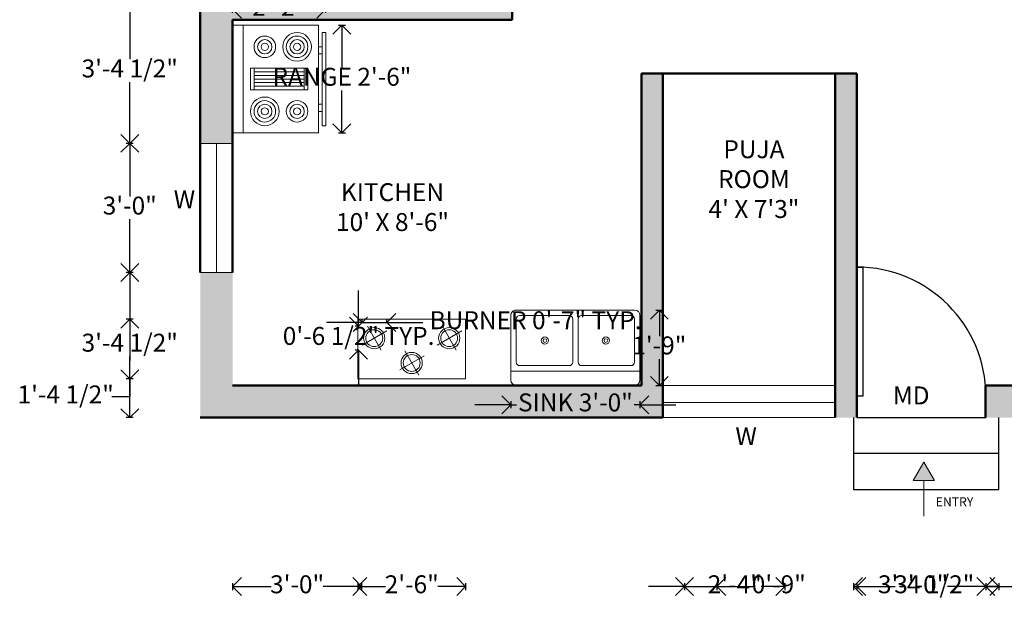
# Model space of a CAD drawing. Units: inches. Extents: x 2691 to 3149, y 584 to 962.
# Tile 1 of 3: x 2691 to 2966, y 584 to 750. Entities that reach past the tile are written whole.
import ezdxf

# ---------------------------------------------------------------- set-up
doc = ezdxf.new("R2010")
doc.units = ezdxf.units.IN
for name, color, linetype, lineweight in [('A-ANNO-DIMS', 2, 'Continuous', 18), ('A-ANNO-SYMB', 252, 'Continuous', 18), ('A-ANNO-TEXT', 159, 'Continuous', 18), ('A-AREA-IDEN', 7, 'Continuous', 25), ('A-DOOR', 4, 'Continuous', 25), ('A-EQPM', 8, 'Continuous', 18), ('A-FLOR-FIXT', 9, 'Continuous', 18), ('A-FLOR-STRS', 7, 'Continuous', 25), ('A-GLAZ', 40, 'Continuous', 18), ('A-WALL', 254, 'Continuous', 50), ('A-WALL-PATT', 252, 'Continuous', 13)]:
    doc.layers.add(name, color=color, linetype=linetype, lineweight=lineweight)
doc.styles.get("Standard").update_dxf_attribs({"font": 'arial.ttf'})
doc.dimstyles.new('ISO-25', dxfattribs={"dimtxt": 5, "dimasz": 5, "dimexe": 1, "dimexo": 1, "dimtad": 0, "dimtih": 1, "dimtoh": 1, "dimdec": 1, "dimlunit": 3, "dimtxsty": 'Standard', "dimblk": 'OPEN90', "dimcen": 2.5, "dimclrd": 1, "dimclre": 1, "dimclrt": 1, "dimadec": 0, "dimazin": 0, "dimtfac": 1, "dimtdec": 1, "dimtmove": 0, "dimatfit": 3, "dimfxl": 1, "dimfxlon": 1, "dimarcsym": 0})

# ---------------------------------------------------------------- blocks, each defined once
blk = doc.blocks.new('*U3')
for p, q in [((0, 0), (0, -6)), ((36, 0), (36, -6))]:
    blk.add_line(p, q)
blk.add_lwpolyline([(0, 0), (0, 36), (1.75, 36), (1.75, 0)], close=True)
blk.add_arc((0, 0), 36, 0, 90)
blk = doc.blocks.new('Sink-double - 36 in top')
for p, q in [((-18, -4), (18, -4)), ((-0.75, -18.5), (-0.75, -6.5)), ((0.75, -6.5), (0.75, -18.5))]:
    blk.add_line(p, q)
for points in [[(-16.5, 0), (16.5, 0)], [(-18, -19.5), (-18, -1.5)], [(18, -1.5), (18, -19.5)], [(-16.5, -18.5), (-16.5, -6.5)], [(-15.5, -5.5), (-1.75, -5.5)], [(1.75, -5.5), (15.5, -5.5)], [(16.5, -6.5), (16.5, -18.5)], [(16.5, -21), (-16.5, -21)], [(-1.75, -19.5), (-15.5, -19.5)], [(15.5, -19.5), (1.75, -19.5)]]:
    blk.add_lwpolyline(points)
for centre, radius in [((-8.5, -12.5), 1), ((-8.5, -12.5), 0.5), ((8.5, -12.5), 1), ((8.5, -12.5), 0.5)]:
    blk.add_circle(centre, radius)
for centre, radius, start, end in [((-16.5, -1.5), 1.5, 90, 180), ((16.5, -1.5), 1.5, 0, 90), ((-15.5, -6.5), 1, 90, 180), ((-1.75, -6.5), 1, 0, 90), ((1.75, -6.5), 1, 90, 180), ((15.5, -6.5), 1, 0, 90), ((-15.5, -18.5), 1, 180, 270), ((-1.75, -18.5), 1, 270, 0), ((1.75, -18.5), 1, 180, 270), ((15.5, -18.5), 1, 270, 0), ((-16.5, -19.5), 1.5, 180, 270), ((16.5, -19.5), 1.5, 270, 0)]:
    blk.add_arc(centre, radius, start, end)
blk = doc.blocks.new('Range-Oven - 30 in top')
for p, q in [((0, -3), (30, -3)), ((12, -6), (18, -6)), ((13, -20), (13, -6)), ((14, -6), (14, -20)), ((15, -20), (15, -6)), ((16, -6), (16, -20)), ((17, -20), (17, -6)), ((18, -20), (12, -20)), ((6, -24), (6, -25)), ((8, -25), (8, -24)), ((22, -25), (22, -24)), ((24, -24), (24, -25))]:
    blk.add_line(p, q)
for points in [[(0, -24), (0, 0), (30, 0), (30, -24)], [(12, -21), (12, -5), (18, -5), (18, -21)], [(2, -26), (2, -25), (28, -25), (28, -26)]]:
    blk.add_lwpolyline(points, close=True)
for centre, radius in [((6, -9), 4), ((6, -9), 3), ((6, -9), 2), ((6, -9), 1), ((24, -9), 3), ((24, -9), 2), ((24, -9), 1), ((6, -18), 3), ((6, -18), 2), ((24, -18), 4), ((24, -18), 3), ((24, -18), 2), ((6, -18), 1), ((24, -18), 1)]:
    blk.add_circle(centre, radius)
blk = doc.blocks.new('COOKTOP-BURNER')
for p, q in [((1.42, 6.72), (5.29, 0)), ((0, 1.45), (6.83, 5.4))]:
    blk.add_line(p, q)
for radius in [2.96, 2.35]:
    blk.add_circle((3.34, 3.38), radius)
blk = doc.blocks.new('_Open90')
at = {"color": 0, "linetype": 'ByBlock', "lineweight": -2}
for p, q in [((0, 0), (-1, 0)), ((-0.5, 0.5), (0, 0)), ((0, 0), (-0.5, -0.5))]:
    blk.add_line(p, q, dxfattribs=at)
blk = doc.blocks.new('*D22')
at = {"layer": 'A-ANNO-DIMS', "color": 1, "lineweight": -2, "transparency": 16777216}
for p, q in [((2781.8, 665.32), (2776.8, 665.32)), ((2786.8, 665.3), (2786.8, 666.32)), ((2786.8, 665.32), (2793.64, 665.32)), ((2793.64, 665.3), (2793.64, 666.32)), ((2798.64, 665.32), (2803.64, 665.32))]:
    blk.add_line(p, q, dxfattribs=at)
at = {"layer": 'Defpoints', "color": 0, "transparency": 16777216}
for p in [(2786.8, 664.3), (2793.64, 665.32), (2793.64, 664.3)]:
    blk.add_point(p, dxfattribs=at)
at = {"layer": 'A-ANNO-DIMS', "color": 1, "lineweight": -2, "transparency": 16777216, "xscale": 5, "yscale": 5, "zscale": 5}
blk.add_blockref('_Open90', (2786.8, 665.32), dxfattribs=at)
at = {"layer": 'A-ANNO-DIMS', "color": 1, "lineweight": -2, "transparency": 16777216, "xscale": 5, "yscale": 5, "zscale": 5, "rotation": 180}
blk.add_blockref('_Open90', (2793.64, 665.32), dxfattribs=at)
at = {"layer": 'A-ANNO-DIMS', "color": 1, "transparency": 16777216, "insert": (2835.11, 665.32), "char_height": 5, "attachment_point": 5}
blk.add_mtext('BURNER 0\'-7" TYP.', dxfattribs=at)
blk = doc.blocks.new('*D23')
at = {"layer": 'A-ANNO-DIMS', "color": 1, "lineweight": -2, "transparency": 16777216}
for p, q in [((2785.78, 669.3), (2785.78, 674.3)), ((2785.8, 664.3), (2784.78, 664.3)), ((2785.78, 664.3), (2785.78, 664.15)), ((2785.8, 657.58), (2784.78, 657.58)), ((2785.78, 657.58), (2785.78, 657.73)), ((2785.78, 652.58), (2785.78, 647.58))]:
    blk.add_line(p, q, dxfattribs=at)
at = {"layer": 'Defpoints', "color": 0, "transparency": 16777216}
for p in [(2785.78, 664.3), (2786.8, 664.3), (2786.8, 657.58)]:
    blk.add_point(p, dxfattribs=at)
at = {"layer": 'A-ANNO-DIMS', "color": 1, "lineweight": -2, "transparency": 16777216, "xscale": 5, "yscale": 5, "zscale": 5}
for p, rotation in [((2785.78, 664.3), 270), ((2785.78, 657.58), 90)]:
    blk.add_blockref('_Open90', p, dxfattribs=dict(at, rotation=rotation))
at = {"layer": 'A-ANNO-DIMS', "color": 1, "transparency": 16777216, "insert": (2785.78, 660.94), "char_height": 5, "attachment_point": 5}
blk.add_mtext('0\'-6 1/2" TYP.', dxfattribs=at)
blk = doc.blocks.new('*D36')
at = {"layer": 'A-ANNO-DIMS', "color": 1, "lineweight": -2, "transparency": 16777216}
for p, q in [((2823.21, 642.4), (2818.21, 642.4)), ((2828.21, 643.4), (2828.21, 641.4)), ((2828.21, 642.4), (2829.83, 642.4)), ((2864.21, 642.4), (2862.59, 642.4)), ((2864.21, 643.4), (2864.21, 641.4)), ((2869.21, 642.4), (2874.21, 642.4))]:
    blk.add_line(p, q, dxfattribs=at)
at = {"layer": 'Defpoints', "color": 0, "transparency": 16777216}
for p in [(2828.21, 647.8), (2864.21, 647.8), (2828.21, 642.4)]:
    blk.add_point(p, dxfattribs=at)
at = {"layer": 'A-ANNO-DIMS', "color": 1, "lineweight": -2, "transparency": 16777216, "xscale": 5, "yscale": 5, "zscale": 5}
blk.add_blockref('_Open90', (2828.21, 642.4), dxfattribs=at)
at = {"layer": 'A-ANNO-DIMS', "color": 1, "lineweight": -2, "transparency": 16777216, "xscale": 5, "yscale": 5, "zscale": 5, "rotation": 180}
blk.add_blockref('_Open90', (2864.21, 642.4), dxfattribs=at)
at = {"layer": 'A-ANNO-DIMS', "color": 1, "transparency": 16777216, "insert": (2846.21, 642.4), "char_height": 5, "attachment_point": 5}
blk.add_mtext('SINK 3\'-0"', dxfattribs=at)
blk = doc.blocks.new('*D37')
at = {"layer": 'A-ANNO-DIMS', "color": 1, "lineweight": -2, "transparency": 16777216}
for p, q in [((2868.61, 668.8), (2870.61, 668.8)), ((2869.61, 663.8), (2869.61, 661.48)), ((2869.61, 652.8), (2869.61, 655.12)), ((2868.61, 647.8), (2870.61, 647.8))]:
    blk.add_line(p, q, dxfattribs=at)
at = {"layer": 'Defpoints', "color": 0, "transparency": 16777216}
for p in [(2864.21, 668.8), (2864.21, 647.8), (2869.61, 647.8)]:
    blk.add_point(p, dxfattribs=at)
at = {"layer": 'A-ANNO-DIMS', "color": 1, "lineweight": -2, "transparency": 16777216, "xscale": 5, "yscale": 5, "zscale": 5}
for p, rotation in [((2869.61, 668.8), 90), ((2869.61, 647.8), 270)]:
    blk.add_blockref('_Open90', p, dxfattribs=dict(at, rotation=rotation))
at = {"layer": 'A-ANNO-DIMS', "color": 1, "transparency": 16777216, "insert": (2869.61, 658.3), "char_height": 5, "attachment_point": 5}
blk.add_mtext('1\'-9"', dxfattribs=at)
blk = doc.blocks.new('*D38')
at = {"layer": 'A-ANNO-DIMS', "color": 1, "lineweight": -2, "transparency": 16777216}
for p, q in [((2780.13, 748.23), (2782.13, 748.23)), ((2781.13, 743.23), (2781.13, 736.44)), ((2781.13, 723.23), (2781.13, 730.02)), ((2780.13, 718.23), (2782.13, 718.23))]:
    blk.add_line(p, q, dxfattribs=at)
at = {"layer": 'Defpoints', "color": 0, "transparency": 16777216}
for p in [(2776.63, 748.23), (2781.13, 748.23), (2776.63, 718.23)]:
    blk.add_point(p, dxfattribs=at)
at = {"layer": 'A-ANNO-DIMS', "color": 1, "lineweight": -2, "transparency": 16777216, "xscale": 5, "yscale": 5, "zscale": 5}
for p, rotation in [((2781.13, 748.23), 90), ((2781.13, 718.23), 270)]:
    blk.add_blockref('_Open90', p, dxfattribs=dict(at, rotation=rotation))
at = {"layer": 'A-ANNO-DIMS', "color": 1, "transparency": 16777216, "insert": (2781.13, 733.23), "char_height": 5, "attachment_point": 5}
blk.add_mtext('RANGE 2\'-6"', dxfattribs=at)
blk = doc.blocks.new('*D39')
at = {"layer": 'A-ANNO-DIMS', "color": 1, "lineweight": -2, "transparency": 16777216}
for p, q in [((2750.63, 751.73), (2750.63, 753.73)), ((2755.63, 752.73), (2756.32, 752.73)), ((2771.63, 752.73), (2770.95, 752.73)), ((2776.63, 751.73), (2776.63, 753.73))]:
    blk.add_line(p, q, dxfattribs=at)
at = {"layer": 'Defpoints', "color": 0, "transparency": 16777216}
for p in [(2750.63, 752.73), (2750.63, 748.23), (2776.63, 748.23)]:
    blk.add_point(p, dxfattribs=at)
at = {"layer": 'A-ANNO-DIMS', "color": 1, "lineweight": -2, "transparency": 16777216, "xscale": 5, "yscale": 5, "zscale": 5, "rotation": 180}
blk.add_blockref('_Open90', (2750.63, 752.73), dxfattribs=at)
at = {"layer": 'A-ANNO-DIMS', "color": 1, "lineweight": -2, "transparency": 16777216, "xscale": 5, "yscale": 5, "zscale": 5}
blk.add_blockref('_Open90', (2776.63, 752.73), dxfattribs=at)
at = {"layer": 'A-ANNO-DIMS', "color": 1, "transparency": 16777216, "insert": (2763.63, 752.73), "char_height": 5, "attachment_point": 5}
blk.add_mtext('2\'-2"', dxfattribs=at)
blk = doc.blocks.new('*D42')
at = {"layer": 'A-ANNO-DIMS', "color": 1, "lineweight": -2, "transparency": 16777216}
for p, q in [((2750.63, 592.67), (2750.63, 590.67)), ((2755.63, 591.67), (2761.36, 591.67)), ((2781.63, 591.67), (2775.9, 591.67)), ((2786.63, 592.67), (2786.63, 590.67))]:
    blk.add_line(p, q, dxfattribs=at)
at = {"layer": 'Defpoints', "color": 0, "transparency": 16777216}
for p in [(2750.63, 929.8), (2786.63, 929.8), (2786.63, 591.67)]:
    blk.add_point(p, dxfattribs=at)
at = {"layer": 'A-ANNO-DIMS', "color": 1, "lineweight": -2, "transparency": 16777216, "xscale": 5, "yscale": 5, "zscale": 5, "rotation": 180}
blk.add_blockref('_Open90', (2750.63, 591.67), dxfattribs=at)
at = {"layer": 'A-ANNO-DIMS', "color": 1, "lineweight": -2, "transparency": 16777216, "xscale": 5, "yscale": 5, "zscale": 5}
blk.add_blockref('_Open90', (2786.63, 591.67), dxfattribs=at)
at = {"layer": 'A-ANNO-DIMS', "color": 1, "transparency": 16777216, "insert": (2768.63, 591.67), "char_height": 5, "attachment_point": 5}
blk.add_mtext('3\'-0"', dxfattribs=at)
blk = doc.blocks.new('*D43')
at = {"layer": 'A-ANNO-DIMS', "color": 1, "lineweight": -2, "transparency": 16777216}
for p, q in [((2871.63, 591.67), (2866.63, 591.67)), ((2876.63, 592.67), (2876.63, 590.67)), ((2876.63, 591.67), (2885.63, 591.67)), ((2885.63, 592.67), (2885.63, 590.67)), ((2890.63, 591.67), (2895.63, 591.67))]:
    blk.add_line(p, q, dxfattribs=at)
at = {"layer": 'Defpoints', "color": 0, "transparency": 16777216}
for p in [(2876.63, 929.8), (2885.63, 929.8), (2885.63, 591.67)]:
    blk.add_point(p, dxfattribs=at)
at = {"layer": 'A-ANNO-DIMS', "color": 1, "lineweight": -2, "transparency": 16777216, "xscale": 5, "yscale": 5, "zscale": 5}
blk.add_blockref('_Open90', (2876.63, 591.67), dxfattribs=at)
at = {"layer": 'A-ANNO-DIMS', "color": 1, "lineweight": -2, "transparency": 16777216, "xscale": 5, "yscale": 5, "zscale": 5, "rotation": 180}
blk.add_blockref('_Open90', (2885.63, 591.67), dxfattribs=at)
at = {"layer": 'A-ANNO-DIMS', "color": 1, "transparency": 16777216, "insert": (2902.9, 591.67), "char_height": 5, "attachment_point": 5}
blk.add_mtext('0\'-9"', dxfattribs=at)
blk = doc.blocks.new('*D44')
at = {"layer": 'A-ANNO-DIMS', "color": 1, "lineweight": -2, "transparency": 16777216}
for p, q in [((2722.98, 679.3), (2720.98, 679.3)), ((2721.98, 674.3), (2721.98, 662.26)), ((2721.98, 643.8), (2721.98, 655.84)), ((2722.98, 638.8), (2720.98, 638.8))]:
    blk.add_line(p, q, dxfattribs=at)
at = {"layer": 'Defpoints', "color": 0, "transparency": 16777216}
for p in [(2721.98, 679.3), (2741.63, 679.3), (2741.63, 638.8)]:
    blk.add_point(p, dxfattribs=at)
at = {"layer": 'A-ANNO-DIMS', "color": 1, "lineweight": -2, "transparency": 16777216, "xscale": 5, "yscale": 5, "zscale": 5}
for p, rotation in [((2721.98, 679.3), 90), ((2721.98, 638.8), 270)]:
    blk.add_blockref('_Open90', p, dxfattribs=dict(at, rotation=rotation))
at = {"layer": 'A-ANNO-DIMS', "color": 1, "transparency": 16777216, "insert": (2721.98, 659.05), "char_height": 5, "attachment_point": 5}
blk.add_mtext('3\'-4 1/2"', dxfattribs=at)
blk = doc.blocks.new('*D45')
at = {"layer": 'A-ANNO-DIMS', "color": 1, "lineweight": -2, "transparency": 16777216}
for p, q in [((2722.98, 715.3), (2720.98, 715.3)), ((2721.98, 710.3), (2721.98, 700.48)), ((2721.98, 684.3), (2721.98, 694.12)), ((2722.98, 679.3), (2720.98, 679.3))]:
    blk.add_line(p, q, dxfattribs=at)
at = {"layer": 'Defpoints', "color": 0, "transparency": 16777216}
for p in [(2721.98, 715.3), (2741.63, 715.3), (2741.63, 679.3)]:
    blk.add_point(p, dxfattribs=at)
at = {"layer": 'A-ANNO-DIMS', "color": 1, "lineweight": -2, "transparency": 16777216, "xscale": 5, "yscale": 5, "zscale": 5}
for p, rotation in [((2721.98, 715.3), 90), ((2721.98, 679.3), 270)]:
    blk.add_blockref('_Open90', p, dxfattribs=dict(at, rotation=rotation))
at = {"layer": 'A-ANNO-DIMS', "color": 1, "transparency": 16777216, "insert": (2721.98, 697.3), "char_height": 5, "attachment_point": 5}
blk.add_mtext('3\'-0"', dxfattribs=at)
blk = doc.blocks.new('*D46')
at = {"layer": 'A-ANNO-DIMS', "color": 1, "lineweight": -2, "transparency": 16777216}
for p, q in [((2722.98, 755.8), (2720.98, 755.8)), ((2721.98, 750.8), (2721.98, 738.76)), ((2721.98, 720.3), (2721.98, 732.34)), ((2722.98, 715.3), (2720.98, 715.3))]:
    blk.add_line(p, q, dxfattribs=at)
at = {"layer": 'Defpoints', "color": 0, "transparency": 16777216}
for p in [(2721.98, 755.8), (2741.63, 755.8), (2741.63, 715.3)]:
    blk.add_point(p, dxfattribs=at)
at = {"layer": 'A-ANNO-DIMS', "color": 1, "lineweight": -2, "transparency": 16777216, "xscale": 5, "yscale": 5, "zscale": 5}
for p, rotation in [((2721.98, 755.8), 90), ((2721.98, 715.3), 270)]:
    blk.add_blockref('_Open90', p, dxfattribs=dict(at, rotation=rotation))
at = {"layer": 'A-ANNO-DIMS', "color": 1, "transparency": 16777216, "insert": (2721.98, 735.55), "char_height": 5, "attachment_point": 5}
blk.add_mtext('3\'-4 1/2"', dxfattribs=at)
blk = doc.blocks.new('*D48')
at = {"layer": 'A-ANNO-DIMS', "color": 1, "lineweight": -2, "transparency": 16777216}
for p, q in [((2960.63, 592.67), (2960.63, 590.67)), ((2965.63, 591.67), (2978.76, 591.67)), ((3006.63, 591.67), (2993.5, 591.67)), ((3011.63, 592.67), (3011.63, 590.67))]:
    blk.add_line(p, q, dxfattribs=at)
at = {"layer": 'Defpoints', "color": 0, "transparency": 16777216}
for p in [(2960.63, 638.8), (3011.63, 638.8), (3011.63, 591.67)]:
    blk.add_point(p, dxfattribs=at)
at = {"layer": 'A-ANNO-DIMS', "color": 1, "lineweight": -2, "transparency": 16777216, "xscale": 5, "yscale": 5, "zscale": 5, "rotation": 180}
blk.add_blockref('_Open90', (2960.63, 591.67), dxfattribs=at)
at = {"layer": 'A-ANNO-DIMS', "color": 1, "lineweight": -2, "transparency": 16777216, "xscale": 5, "yscale": 5, "zscale": 5}
blk.add_blockref('_Open90', (3011.63, 591.67), dxfattribs=at)
at = {"layer": 'A-ANNO-DIMS', "color": 1, "transparency": 16777216, "insert": (2986.13, 591.67), "char_height": 5, "attachment_point": 5}
blk.add_mtext('4\'-3"', dxfattribs=at)
blk = doc.blocks.new('*D49')
at = {"layer": 'A-ANNO-DIMS', "color": 1, "lineweight": -2, "transparency": 16777216}
for p, q in [((2924.63, 592.67), (2924.63, 590.67)), ((2929.63, 591.67), (2935.36, 591.67)), ((2955.63, 591.67), (2949.9, 591.67)), ((2960.63, 592.67), (2960.63, 590.67))]:
    blk.add_line(p, q, dxfattribs=at)
at = {"layer": 'Defpoints', "color": 0, "transparency": 16777216}
for p in [(2924.63, 638.8), (2960.63, 638.8), (2960.63, 591.67)]:
    blk.add_point(p, dxfattribs=at)
at = {"layer": 'A-ANNO-DIMS', "color": 1, "lineweight": -2, "transparency": 16777216, "xscale": 5, "yscale": 5, "zscale": 5, "rotation": 180}
blk.add_blockref('_Open90', (2924.63, 591.67), dxfattribs=at)
at = {"layer": 'A-ANNO-DIMS', "color": 1, "lineweight": -2, "transparency": 16777216, "xscale": 5, "yscale": 5, "zscale": 5}
blk.add_blockref('_Open90', (2960.63, 591.67), dxfattribs=at)
at = {"layer": 'A-ANNO-DIMS', "color": 1, "transparency": 16777216, "insert": (2942.63, 591.67), "char_height": 5, "attachment_point": 5}
blk.add_mtext('3\'-0"', dxfattribs=at)
blk = doc.blocks.new('*D50')
at = {"layer": 'A-ANNO-DIMS', "color": 1, "lineweight": -2, "transparency": 16777216}
for p, q in [((2876.63, 592.67), (2876.63, 590.67)), ((2881.63, 591.67), (2883.32, 591.67)), ((2899.63, 591.67), (2897.95, 591.67)), ((2904.63, 592.67), (2904.63, 590.67))]:
    blk.add_line(p, q, dxfattribs=at)
at = {"layer": 'Defpoints', "color": 0, "transparency": 16777216}
for p in [(2876.63, 857.8), (2904.63, 857.8), (2904.63, 591.67)]:
    blk.add_point(p, dxfattribs=at)
at = {"layer": 'A-ANNO-DIMS', "color": 1, "lineweight": -2, "transparency": 16777216, "xscale": 5, "yscale": 5, "zscale": 5, "rotation": 180}
blk.add_blockref('_Open90', (2876.63, 591.67), dxfattribs=at)
at = {"layer": 'A-ANNO-DIMS', "color": 1, "lineweight": -2, "transparency": 16777216, "xscale": 5, "yscale": 5, "zscale": 5}
blk.add_blockref('_Open90', (2904.63, 591.67), dxfattribs=at)
at = {"layer": 'A-ANNO-DIMS', "color": 1, "transparency": 16777216, "insert": (2890.63, 591.67), "char_height": 5, "attachment_point": 5}
blk.add_mtext('2\'-4"', dxfattribs=at)
blk = doc.blocks.new('*D54')
at = {"layer": 'A-ANNO-DIMS', "color": 1, "lineweight": -2, "transparency": 16777216}
for p, q in [((2923.71, 592.67), (2923.71, 590.67)), ((2928.71, 591.67), (2930.89, 591.67)), ((2959.26, 591.67), (2957.08, 591.67)), ((2964.26, 592.67), (2964.26, 590.67))]:
    blk.add_line(p, q, dxfattribs=at)
at = {"layer": 'Defpoints', "color": 0, "transparency": 16777216}
for p in [(2923.71, 618.8), (2964.26, 618.8), (2964.26, 591.67)]:
    blk.add_point(p, dxfattribs=at)
at = {"layer": 'A-ANNO-DIMS', "color": 1, "lineweight": -2, "transparency": 16777216, "xscale": 5, "yscale": 5, "zscale": 5, "rotation": 180}
blk.add_blockref('_Open90', (2923.71, 591.67), dxfattribs=at)
at = {"layer": 'A-ANNO-DIMS', "color": 1, "lineweight": -2, "transparency": 16777216, "xscale": 5, "yscale": 5, "zscale": 5}
blk.add_blockref('_Open90', (2964.26, 591.67), dxfattribs=at)
at = {"layer": 'A-ANNO-DIMS', "color": 1, "transparency": 16777216, "insert": (2943.98, 591.67), "char_height": 5, "attachment_point": 5}
blk.add_mtext('3\'-4 1/2"', dxfattribs=at)
blk = doc.blocks.new('*D55')
at = {"layer": 'A-ANNO-DIMS', "color": 1, "lineweight": -2, "transparency": 16777216}
for p, q in [((3120.3, 638.8), (3122.3, 638.8)), ((3121.3, 633.8), (3121.3, 631.98)), ((3121.3, 623.8), (3121.3, 625.62)), ((3120.3, 618.8), (3122.3, 618.8))]:
    blk.add_line(p, q, dxfattribs=at)
at = {"layer": 'Defpoints', "color": 0, "transparency": 16777216}
for p in [(2964.26, 638.8), (3121.3, 638.8), (2964.26, 618.8)]:
    blk.add_point(p, dxfattribs=at)
at = {"layer": 'A-ANNO-DIMS', "color": 1, "lineweight": -2, "transparency": 16777216, "xscale": 5, "yscale": 5, "zscale": 5}
for p, rotation in [((3121.3, 638.8), 90), ((3121.3, 618.8), 270)]:
    blk.add_blockref('_Open90', p, dxfattribs=dict(at, rotation=rotation))
at = {"layer": 'A-ANNO-DIMS', "color": 1, "transparency": 16777216, "insert": (3121.3, 628.8), "char_height": 5, "attachment_point": 5}
blk.add_mtext('1\'-8"', dxfattribs=at)
blk = doc.blocks.new('*D56')
at = {"layer": 'A-ANNO-DIMS', "color": 1, "lineweight": -2, "transparency": 16777216}
for p, q in [((2785.56, 592.67), (2785.56, 590.67)), ((2790.56, 591.67), (2793.28, 591.67)), ((2810.62, 591.67), (2807.91, 591.67)), ((2815.62, 592.67), (2815.62, 590.67))]:
    blk.add_line(p, q, dxfattribs=at)
at = {"layer": 'Defpoints', "color": 0, "transparency": 16777216}
for p in [(2785.56, 649.62), (2815.62, 649.62), (2815.62, 591.67)]:
    blk.add_point(p, dxfattribs=at)
at = {"layer": 'A-ANNO-DIMS', "color": 1, "lineweight": -2, "transparency": 16777216, "xscale": 5, "yscale": 5, "zscale": 5, "rotation": 180}
blk.add_blockref('_Open90', (2785.56, 591.67), dxfattribs=at)
at = {"layer": 'A-ANNO-DIMS', "color": 1, "lineweight": -2, "transparency": 16777216, "xscale": 5, "yscale": 5, "zscale": 5}
blk.add_blockref('_Open90', (2815.62, 591.67), dxfattribs=at)
at = {"layer": 'A-ANNO-DIMS', "color": 1, "transparency": 16777216, "insert": (2800.59, 591.67), "char_height": 5, "attachment_point": 5}
blk.add_mtext('2\'-6"', dxfattribs=at)
blk = doc.blocks.new('*D57')
at = {"layer": 'A-ANNO-DIMS', "color": 1, "lineweight": -2, "transparency": 16777216}
for p, q in [((2722.98, 666.25), (2720.98, 666.25)), ((2721.98, 661.25), (2721.98, 654.62)), ((2722.98, 649.62), (2720.98, 649.62)), ((2721.98, 649.62), (2721.98, 644.62)), ((2721.98, 644.62), (2716.98, 644.62))]:
    blk.add_line(p, q, dxfattribs=at)
at = {"layer": 'Defpoints', "color": 0, "transparency": 16777216}
for p in [(2785.56, 666.25), (2721.98, 649.62), (2785.56, 649.62)]:
    blk.add_point(p, dxfattribs=at)
at = {"layer": 'A-ANNO-DIMS', "color": 1, "lineweight": -2, "transparency": 16777216, "xscale": 5, "yscale": 5, "zscale": 5}
for p, rotation in [((2721.98, 666.25), 90), ((2721.98, 649.62), 270)]:
    blk.add_blockref('_Open90', p, dxfattribs=dict(at, rotation=rotation))
at = {"layer": 'A-ANNO-DIMS', "color": 1, "transparency": 16777216, "insert": (2704.12, 644.62), "char_height": 5, "attachment_point": 5}
blk.add_mtext('1\'-4 1/2"', dxfattribs=at)

msp = doc.modelspace()

# ---------------------------------------------------------------- hatches: boundary and pattern name
at = {"layer": 'A-ANNO-SYMB'}
h = msp.add_hatch(color=256, dxfattribs=at)
h.dxf.hatch_style = 1
h.paths.add_polyline_path([(2943.34, 626.41), (2940.34, 621.22), (2943.34, 621.22), (2946.34, 621.22)])
at = {"layer": 'A-WALL-PATT'}
h = msp.add_hatch(color=256, dxfattribs=at)
h.dxf.hatch_style = 1
h.paths.add_polyline_path([(2786.63, 938.8), (2741.63, 938.8), (2741.63, 803.8), (2822.63, 803.8), (2822.63, 785.8), (2828.63, 785.8), (2828.63, 803.8), (2876.63, 803.8), (2876.63, 809.8), (2870.63, 809.8), (2834.63, 809.8), (2750.63, 809.8), (2750.63, 929.8), (2786.63, 929.8)])
h.paths.add_polyline_path([(2885.63, 938.8), (2834.63, 938.8), (2834.63, 929.8), (2840.63, 929.8), (2870.63, 929.8), (2870.63, 885.8), (2876.63, 885.8), (2876.63, 929.8), (2885.63, 929.8)])
h.paths.add_polyline_path([(2933.63, 938.8), (2909.63, 938.8), (2909.63, 929.8), (2918.63, 929.8), (2918.63, 908.89), (2918.64, 908.89), (2918.63, 925.2), (2912.41, 925.19), (2912.43, 908.88), (2918.63, 908.89), (2918.63, 925.2), (2918.63, 925.2), (2918.64, 908.89), (2918.63, 857.8), (2870.63, 857.8), (2870.63, 845.8), (2876.63, 845.8), (2876.63, 851.8), (2966.63, 851.8), (2966.63, 845.8), (2972.63, 845.8), (2972.63, 857.8), (2924.63, 857.8), (2924.63, 929.8), (2933.63, 929.8)])
h.paths.add_polyline_path([(2917.85, 923.84), (2917.86, 910.44, -0.414214), (2917.28, 909.66), (2913.98, 909.66, -0.414214), (2913.2, 910.24), (2913.19, 923.64, -0.414214), (2913.77, 924.42), (2917.07, 924.42, -0.414214)], flags=16)
h.paths.add_polyline_path([(3008.63, 938.8), (2957.63, 938.8), (2957.63, 929.8), (2966.63, 929.8), (2966.63, 885.8), (2972.63, 885.8), (2972.63, 929.8), (3008.63, 929.8)])
h.paths.add_polyline_path([(3101.63, 938.8), (3056.63, 938.8), (3056.63, 929.8), (3063.83, 929.8), (3092.63, 929.8), (3092.63, 809.8), (2966.63, 809.8), (2966.63, 803.8), (2972.63, 803.8), (2972.63, 797.8), (2978.63, 797.8), (2978.63, 803.8), (3092.63, 803.8), (3092.63, 749.8), (3101.63, 749.8)])
h.paths.add_polyline_path([(2828.63, 757.8), (2822.63, 757.8), (2822.63, 755.8), (2741.63, 755.8), (2741.63, 715.3), (2750.63, 715.3), (2750.63, 749.8), (2828.63, 749.8)])
h.paths.add_polyline_path([(2870.63, 734.8), (2864.63, 734.8), (2864.63, 647.8), (2750.63, 647.8), (2750.63, 679.3), (2741.63, 679.3), (2741.63, 638.8), (2870.63, 638.8)])
h.paths.add_polyline_path([(2924.63, 680.8), (2924.63, 734.8), (2918.63, 734.8), (2918.63, 638.8), (2924.63, 638.8), (2924.63, 644.8)])
h.paths.add_polyline_path([(3011.63, 647.8), (2978.63, 647.8), (2978.63, 761.8), (2972.63, 761.8), (2972.63, 647.8), (2960.51, 647.8, -0.020861), (2960.63, 644.8), (2960.63, 638.8), (3011.63, 638.8)])
h.paths.add_polyline_path([(3101.63, 701.8), (3092.63, 701.8), (3092.63, 647.8), (3059.63, 647.8), (3059.63, 638.8), (3101.63, 638.8)])

# ---------------------------------------------------------------- linework, layer by layer
at = {"layer": 'A-ANNO-SYMB'}
for p, q in [((2940.34, 621.22), (2943.34, 626.41)), ((2946.34, 621.22), (2943.34, 626.41)), ((2943.34, 621.22), (2940.34, 621.22)), ((2943.34, 611.32), (2943.34, 621.22)), ((2943.34, 621.22), (2946.34, 621.22))]:
    msp.add_line(p, q, dxfattribs=at)
at = {"layer": 'A-DOOR'}
msp.add_line((2924.63, 638.8), (2960.63, 638.8), dxfattribs=at)
at = {"layer": 'A-EQPM'}
msp.add_lwpolyline([(2785.56, 666.25), (2815.62, 666.25), (2815.62, 649.62), (2785.56, 649.62)], close=True, dxfattribs=at)
at = {"layer": 'A-FLOR-STRS'}
for p, q in [((2923.71, 638.8), (2923.71, 618.8)), ((2964.26, 618.8), (2964.26, 638.8)), ((2964.26, 628.8), (2923.71, 628.8)), ((2923.71, 618.8), (2964.26, 618.8))]:
    msp.add_line(p, q, dxfattribs=at)
at = {"layer": 'A-GLAZ'}
for p, q in [((2750.63, 715.3), (2741.63, 715.3)), ((2746.13, 679.3), (2746.13, 715.3)), ((2750.63, 679.3), (2741.63, 679.3)), ((2870.63, 647.8), (2918.63, 647.8)), ((2870.63, 643.02), (2918.63, 643.02)), ((2870.63, 638.8), (2918.63, 638.8))]:
    msp.add_line(p, q, dxfattribs=at)
at = {"layer": 'A-WALL'}
for p, q in [((2828.63, 757.8), (2828.63, 749.8)), ((2741.63, 755.8), (2741.63, 679.3)), ((2750.63, 749.8), (2828.63, 749.8)), ((2750.63, 749.8), (2750.63, 679.3)), ((2864.63, 734.8), (2864.63, 647.8)), ((2864.63, 734.8), (2924.63, 734.8)), ((2870.63, 734.8), (2870.63, 638.8)), ((2918.63, 734.8), (2918.63, 638.8)), ((2924.63, 734.8), (2924.63, 638.8)), ((2750.63, 647.8), (2864.63, 647.8)), ((2960.51, 647.8), (2972.63, 647.8)), ((2960.51, 647.8), (2960.51, 638.8)), ((2741.63, 638.8), (2870.63, 638.8))]:
    msp.add_line(p, q, dxfattribs=at)

# ---------------------------------------------------------------- block references
at = {"layer": 'A-DOOR'}
msp.add_blockref('*U3', (2924.63, 644.8), dxfattribs=at)
at = {"layer": 'A-EQPM', "rotation": 89.99999999999999}
msp.add_blockref('Range-Oven - 30 in top', (2750.63, 718.23), dxfattribs=at)
at = {"layer": 'A-EQPM'}
for p in [(2786.8, 657.58), (2807.7, 657.58), (2797.24, 650.67)]:
    msp.add_blockref('COOKTOP-BURNER', p, dxfattribs=at)
at = {"layer": 'A-FLOR-FIXT', "rotation": 180}
msp.add_blockref('Sink-double - 36 in top', (2846.21, 647.8), dxfattribs=at)

# ---------------------------------------------------------------- texts
at = {"layer": 'A-ANNO-TEXT', "attachment_point": 1}
for s, width, insert, char_height in [('\\pxqc;{W}', 11.2162, (2731.62, 702.2), 5), ('\\pxqc;{MD}', 11.2162, (2934.22, 647.5), 5), ('\\pxqc;{W}', 11.2162, (2888.19, 636.14), 5), ('\\pxqc;{ENTRY}', 12.4683, (2945.67, 616.59), 2.5)]:
    msp.add_mtext_dynamic_manual_height_columns(s, width=width, gutter_width=12.5, heights=[0], dxfattribs=dict(at, insert=insert, char_height=char_height))
at = {"layer": 'A-AREA-IDEN', "char_height": 5, "attachment_point": 1}
for s, insert in [('\\pxqc;PUJA \\PROOM\\P4\' X 7\'3"', (2870.63, 716.16)), ('\\pxqc;KITCHEN\\P10\' X 8\'-6"', (2769.88, 704.19))]:
    msp.add_mtext_dynamic_manual_height_columns(s, width=50.6943, gutter_width=12.5, heights=[0], dxfattribs=dict(at, insert=insert))

# ---------------------------------------------------------------- dimensions: what is measured, and where the dimension line sits
at = {"layer": 'A-ANNO-DIMS'}
for base, p1, p2, picture, middle in [((2786.63, 591.67), (2750.63, 929.8), (2786.63, 929.8), '*D42', (2768.63, 591.67)), ((2885.63, 591.67), (2876.63, 929.8), (2885.63, 929.8), '*D43', (2902.9, 591.67)), ((2904.63, 591.67), (2876.63, 857.8), (2904.63, 857.8), '*D50', (2890.63, 591.67)), ((2815.62, 591.67), (2785.56, 649.62), (2815.62, 649.62), '*D56', (2800.59, 591.67)), ((2960.63, 591.67), (2924.63, 638.8), (2960.63, 638.8), '*D49', (2942.63, 591.67)), ((3011.63, 591.67), (2960.63, 638.8), (3011.63, 638.8), '*D48', (2986.13, 591.67)), ((2964.2613, 591.6737), (2923.7075, 618.7981), (2964.2613, 618.7981), '*D54', (2943.9844, 591.6737))]:
    dim = msp.add_linear_dim(base=base, p1=p1, p2=p2, dimstyle='ISO-25', override={"dimdec": 1, "dimlfac": 1, "dimrnd": 0, "dimzin": 1, "dimdsep": 46, "dimlunit": 4, "dimfrac": 2}, dxfattribs=at)
    dim.commit()
    dim.dimension.update_dxf_attribs({"geometry": picture, "text_midpoint": middle})
for base, p1, p2, angle, picture, middle in [((2721.98, 755.8), (2741.63, 715.3), (2741.63, 755.8), 90, '*D46', (2721.98, 735.55)), ((2750.63, 752.73), (2776.63, 748.23), (2750.63, 748.23), 180, '*D39', (2763.63, 752.73)), ((2721.98, 715.3), (2741.63, 679.3), (2741.63, 715.3), 90, '*D45', (2721.98, 697.3)), ((2721.98, 679.3), (2741.63, 638.8), (2741.63, 679.3), 90, '*D44', (2721.98, 659.05)), ((2869.61, 647.8), (2864.21, 668.8), (2864.21, 647.8), 270, '*D37', (2869.61, 658.3)), ((2721.98, 649.62), (2785.56, 666.25), (2785.56, 649.62), 90, '*D57', (2704.12, 644.62)), ((3121.3, 638.8), (2964.26, 618.8), (2964.26, 638.8), 90, '*D55', (3121.3, 628.8))]:
    dim = msp.add_linear_dim(base=base, p1=p1, p2=p2, angle=angle, dimstyle='ISO-25', override={"dimdec": 1, "dimlfac": 1, "dimrnd": 0, "dimzin": 1, "dimdsep": 46, "dimlunit": 4, "dimfrac": 2}, dxfattribs=at)
    dim.commit()
    dim.dimension.update_dxf_attribs({"geometry": picture, "text_midpoint": middle})
for base, p1, p2, angle, text, picture, middle in [((2781.13, 748.23), (2776.63, 718.23), (2776.63, 748.23), 90, 'RANGE <>', '*D38', (2781.13, 733.23)), ((2785.78, 664.3), (2786.8, 657.58), (2786.8, 664.3), 90, '<> TYP.', '*D23', (2785.78, 660.94)), ((2828.21, 642.4), (2864.21, 647.8), (2828.21, 647.8), 180, 'SINK <>', '*D36', (2846.21, 642.4))]:
    dim = msp.add_linear_dim(base=base, p1=p1, p2=p2, angle=angle, text=text, dimstyle='ISO-25', override={"dimdec": 1, "dimlfac": 1, "dimrnd": 0, "dimzin": 1, "dimdsep": 46, "dimlunit": 4, "dimfrac": 2}, dxfattribs=at)
    dim.commit()
    dim.dimension.update_dxf_attribs({"geometry": picture, "text_midpoint": middle})
dim = msp.add_linear_dim(base=(2793.64, 665.32), p1=(2786.8, 664.3), p2=(2793.64, 664.3), text='BURNER <> TYP.', dimstyle='ISO-25', override={"dimdec": 1, "dimlfac": 1, "dimrnd": 0, "dimzin": 1, "dimdsep": 46, "dimlunit": 4, "dimfrac": 2}, dxfattribs=at)
dim.commit()
dim.dimension.update_dxf_attribs({"geometry": '*D22', "text_midpoint": (2835.11, 665.32)})

doc.saveas('drawing.dxf')
